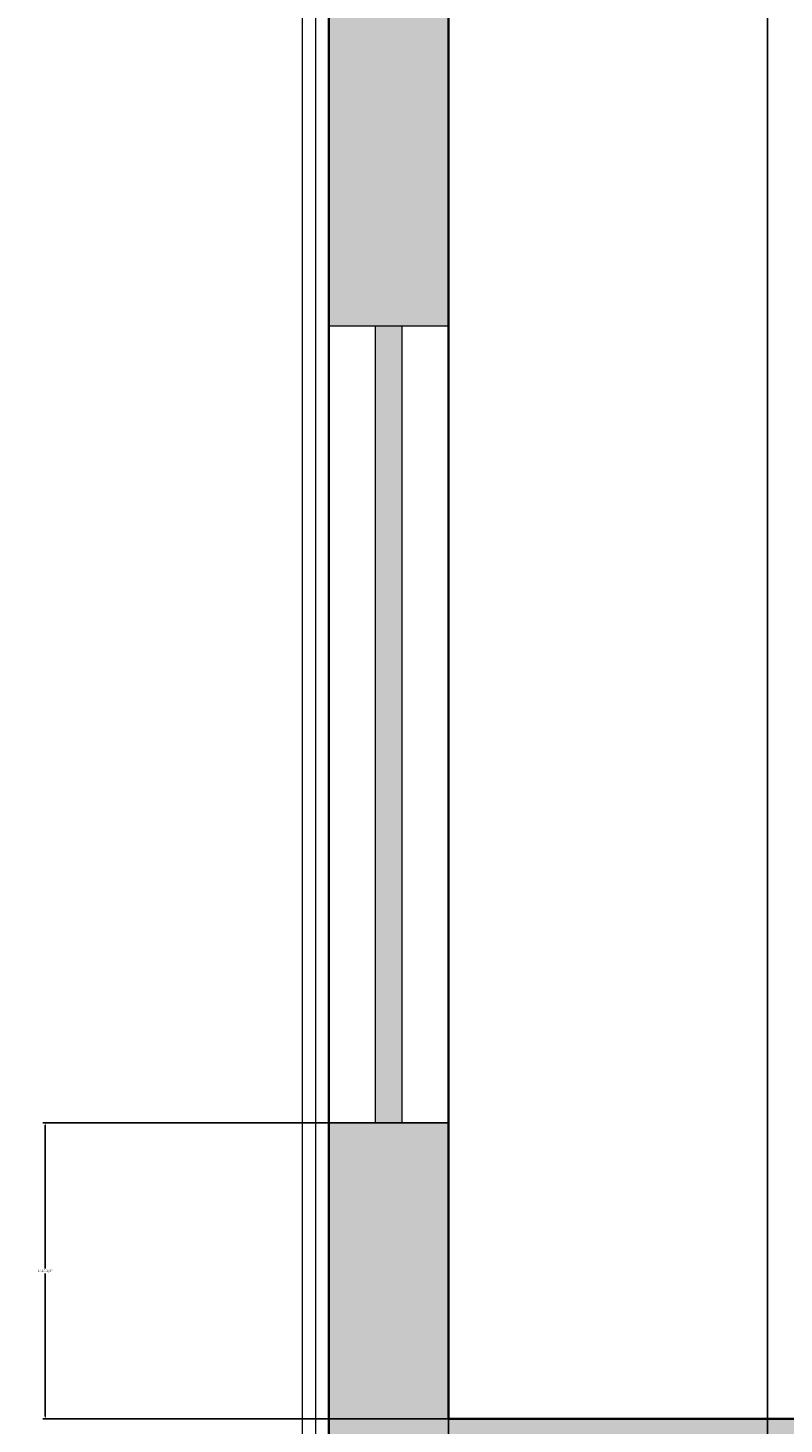
# Model space of a CAD drawing. Units: inches. Extents: x 311 to 815, y -527 to 136.
# Tile 3 of 21: x 388 to 445, y -474 to -368. Entities that reach past the tile are written whole.
import ezdxf

# ---------------------------------------------------------------- set-up
doc = ezdxf.new("R2010")
doc.units = ezdxf.units.IN
doc.header["$MEASUREMENT"] = 0
for name, color, linetype, lineweight in [('A-ANNO-DIMS', 1, 'Continuous', 18), ('A-FLOR-EDGE', 1, 'Continuous', 18), ('A-GLAZ-PATT', 5, 'Continuous', 13), ('A-WALL-PATT', 242, 'Continuous', 13), ('wall', 1, 'Continuous', 35), ('win', 5, 'Continuous', 18)]:
    doc.layers.add(name, color=color, linetype=linetype, lineweight=lineweight)
doc.styles.get("Standard").update_dxf_attribs({"font": 'arial.ttf'})
doc.dimstyles.get("Standard").update_dxf_attribs({"dimtxt": 0.18, "dimasz": 0.18, "dimexe": 0.18, "dimexo": 0.0625, "dimgap": 0.09, "dimtad": 0, "dimtih": 1, "dimtoh": 1, "dimdec": 1, "dimzin": 0, "dimdsep": 46, "dimlunit": 4, "dimtxsty": 'Standard', "dimcen": 0.09, "dimadec": 0, "dimazin": 0, "dimtfac": 1, "dimtdec": 1, "dimtofl": 0, "dimtmove": 0, "dimatfit": 3, "dimfxl": 1, "dimtolj": 1, "dimtzin": 0, "dimarcsym": 0})

# ---------------------------------------------------------------- blocks, each defined once
blk = doc.blocks.new('_ArchTick')
at = {"color": 0, "linetype": 'ByBlock', "const_width": 0.15}
blk.add_lwpolyline([(-0.5, -0.5), (0.5, 0.5)], dxfattribs=at)
blk = doc.blocks.new('_Oblique')
at = {"color": 0, "linetype": 'ByBlock', "lineweight": -2}
blk.add_line((-0.5, -0.5), (0.5, 0.5), dxfattribs=at)
blk = doc.blocks.new('*D3')
at = {"layer": 'A-ANNO-DIMS', "color": 0, "lineweight": -2, "transparency": 16777216}
for p, q in [((377.54, 21.87), (377.54, -221.61)), ((377.54, -482.13), (377.54, -238.65))]:
    blk.add_line(p, q, dxfattribs=at)
at = {"layer": 'Defpoints', "color": 0, "transparency": 16777216}
for p in [(410.32, 21.87), (377.54, -482.13), (410.32, -482.13)]:
    blk.add_point(p, dxfattribs=at)
at = {"layer": 'A-ANNO-DIMS', "color": 0, "lineweight": -2, "transparency": 16777216, "xscale": 9, "yscale": 9, "zscale": 9}
for name, p, rotation in [('_ArchTick', (377.54, 21.87), 90), ('_Oblique', (377.54, -482.13), 270)]:
    blk.add_blockref(name, p, dxfattribs=dict(at, rotation=rotation))
at = {"layer": 'A-ANNO-DIMS', "color": 0, "transparency": 16777216, "insert": (377.54, -230.13), "char_height": 9, "attachment_point": 5}
blk.add_mtext("\\A1;42'", dxfattribs=at)
blk = doc.blocks.new('WIN-60IN')
for p, q in [((9, 60), (0, 60)), ((3.5, 0), (3.5, 60)), ((5.5, 0), (5.5, 60)), ((9, 0), (0, 0))]:
    blk.add_line(p, q)
blk = doc.blocks.new('*D44')
at = {"layer": 'A-ANNO-DIMS', "color": 0, "lineweight": -2, "transparency": 16777216}
for p, q in [((419.26, -450.84), (388.79, -450.84)), ((388.97, -451.02), (388.97, -461.8)), ((388.97, -472.95), (388.97, -462.17)), ((419.26, -473.13), (388.79, -473.13))]:
    blk.add_line(p, q, dxfattribs=at)
at = {"layer": 'A-ANNO-DIMS', "color": 0, "transparency": 16777216}
for points in [[(388.94, -451.02), (389, -451.02), (388.97, -450.84)], [(388.94, -472.95), (389, -472.95), (388.97, -473.13)]]:
    blk.add_solid(points, dxfattribs=at)
at = {"layer": 'Defpoints', "color": 0, "transparency": 16777216}
for p in [(388.97, -450.84), (419.32, -450.84), (419.32, -473.13)]:
    blk.add_point(p, dxfattribs=at)
at = {"layer": 'A-ANNO-DIMS', "color": 0, "transparency": 16777216, "insert": (388.97, -461.98), "char_height": 0.18, "attachment_point": 5}
blk.add_mtext('\\A1;1\'-10 1/2"', dxfattribs=at)
blk = doc.blocks.new('*D54')
at = {"layer": 'A-ANNO-DIMS', "color": 0, "lineweight": -2, "transparency": 16777216}
for p, q in [((419.32, -335.63), (419.32, -526.66)), ((443.32, -348.19), (443.32, -526.66)), ((419.5, -526.48), (430.99, -526.48)), ((443.14, -526.48), (431.65, -526.48))]:
    blk.add_line(p, q, dxfattribs=at)
at = {"layer": 'A-ANNO-DIMS', "color": 0, "transparency": 16777216}
for points in [[(419.5, -526.45), (419.5, -526.51), (419.32, -526.48)], [(443.14, -526.45), (443.14, -526.51), (443.32, -526.48)]]:
    blk.add_solid(points, dxfattribs=at)
at = {"layer": 'Defpoints', "color": 0, "transparency": 16777216}
for p in [(419.32, -335.57), (443.32, -348.13), (443.32, -526.48)]:
    blk.add_point(p, dxfattribs=at)
at = {"layer": 'A-ANNO-DIMS', "color": 0, "transparency": 16777216, "insert": (431.32, -526.48), "char_height": 0.18, "attachment_point": 5}
blk.add_mtext('\\A1;2\'-0"', dxfattribs=at)

msp = doc.modelspace()

# ---------------------------------------------------------------- hatches: boundary and pattern name
at = {"layer": 'A-GLAZ-PATT'}
h = msp.add_hatch(color=256, dxfattribs=at)
h.dxf.hatch_style = 1
h.paths.add_polyline_path([(415.82, -202.13), (413.82, -202.13), (413.82, -262.13), (415.82, -262.13)])
h.paths.add_polyline_path([(415.82, -390.84), (413.82, -390.84), (413.82, -450.84), (415.82, -450.84)])
h.paths.add_polyline_path([(415.82, -311.57), (413.82, -311.57), (413.82, -335.57), (415.82, -335.57)])
h.paths.add_polyline_path([(509.32, -476.63), (449.32, -476.63), (449.32, -478.63), (509.32, -478.63)])
h.paths.add_polyline_path([(606.82, -476.63), (582.82, -476.63), (582.82, -478.63), (606.82, -478.63)])
h.paths.add_polyline_path([(678.82, -476.63), (654.82, -476.63), (654.82, -478.63), (678.82, -478.63)])
h.paths.add_polyline_path([(718.82, -385.13), (716.82, -385.13), (716.82, -445.13), (718.82, -445.13)])
h.paths.add_polyline_path([(718.82, -262.63), (716.82, -262.63), (716.82, -322.63), (718.82, -322.63)])
h.paths.add_polyline_path([(718.82, -140.13), (716.82, -140.13), (716.82, -200.13), (718.82, -200.13)])
h.paths.add_polyline_path([(718.82, -18.13), (716.82, -18.13), (716.82, -42.13), (718.82, -42.13)])
h.paths.add_polyline_path([(686.82, 18.37), (626.82, 18.37), (626.82, 16.37), (686.82, 16.37)])
h.paths.add_polyline_path([(581.82, 18.37), (557.82, 18.37), (557.82, 16.37), (581.82, 16.37)])
h.paths.add_polyline_path([(509.32, 18.37), (449.32, 18.37), (449.32, 16.37), (509.32, 16.37)])
at = {"layer": 'A-WALL-PATT'}
h = msp.add_hatch(color=256, dxfattribs=at)
h.dxf.hatch_style = 1
h.paths.add_polyline_path([(557.82, 21.87), (509.32, 21.87), (509.32, 12.87), (539.32, 12.87), (539.32, -112.13), (548.32, -112.13), (548.32, -58.63), (557.82, -58.63), (557.82, -49.63), (548.32, -49.63), (548.32, 12.87), (557.82, 12.87)])
h.paths.add_polyline_path([(449.32, 21.87), (410.32, 21.87), (410.32, -15.13), (419.32, -15.13), (419.32, 12.87), (449.32, 12.87)])
h.paths.add_polyline_path([(626.82, 21.87), (581.82, 21.87), (581.82, 12.87), (591.32, 12.87), (591.32, -49.63), (581.82, -49.63), (581.82, -58.63), (591.32, -58.63), (591.32, -112.13), (600.32, -112.13), (600.32, 12.87), (626.82, 12.87)])
h.paths.add_polyline_path([(722.32, 21.87), (686.82, 21.87), (686.82, 12.87), (713.32, 12.87), (713.32, -18.13), (722.32, -18.13)])
h.paths.add_polyline_path([(722.32, -42.13), (713.32, -42.13), (713.32, -73.13), (722.32, -73.13)])
h.paths.add_polyline_path([(501.32, -103.13), (419.32, -103.13), (419.32, -75.13), (410.32, -75.13), (410.32, -126.63), (419.32, -126.63), (419.32, -112.13), (492.32, -112.13), (492.32, -143.13), (501.32, -143.13)])
h.paths.add_polyline_path([(548.32, -165.13), (419.32, -165.13), (419.32, -150.63), (410.32, -150.63), (410.32, -202.13), (419.32, -202.13), (419.32, -174.13), (548.32, -174.13)])
h.paths.add_polyline_path([(722.32, -103.13), (636.32, -103.13), (636.32, -112.13), (713.32, -112.13), (713.32, -140.13), (722.32, -140.13)])
h.paths.add_polyline_path([(548.32, -210.13), (539.32, -210.13), (539.32, -290.13), (419.32, -290.13), (419.32, -262.13), (410.32, -262.13), (410.32, -311.57), (419.32, -311.57), (419.32, -299.13), (469.32, -299.13), (469.32, -348.13), (443.32, -348.13), (443.32, -357.13), (478.32, -357.13), (478.32, -299.13), (548.32, -299.13)])
h.paths.add_polyline_path([(722.32, -200.13), (713.32, -200.13), (713.32, -228.13), (609.32, -228.13), (609.32, -237.13), (713.32, -237.13), (713.32, -262.63), (722.32, -262.63)])
h.paths.add_polyline_path([(722.32, -322.63), (713.32, -322.63), (713.32, -348.13), (633.32, -348.13), (633.32, -357.13), (713.32, -357.13), (713.32, -385.13), (722.32, -385.13)])
h.paths.add_polyline_path([(419.32, -335.57), (410.32, -335.57), (410.32, -390.84), (419.32, -390.84)])
h.paths.add_polyline_path([(419.32, -450.84), (410.32, -450.84), (410.32, -482.13), (449.32, -482.13), (449.32, -473.13), (419.32, -473.13)])
h.paths.add_polyline_path([(582.82, -473.13), (548.32, -473.13), (548.32, -348.13), (539.32, -348.13), (539.32, -473.13), (509.32, -473.13), (509.32, -482.13), (582.82, -482.13)])
h.paths.add_polyline_path([(722.32, -445.13), (713.32, -445.13), (713.32, -473.13), (678.82, -473.13), (678.82, -482.13), (722.32, -482.13)])

# ---------------------------------------------------------------- linework, layer by layer
at = {"layer": 'A-FLOR-EDGE'}
for p, q in [((408.32, -484.13), (408.32, 23.87)), ((409.32, -483.13), (409.32, 22.87))]:
    msp.add_line(p, q, dxfattribs=at)
at = {"layer": 'wall'}
for p, q in [((410.32, -482.13), (410.32, 21.87)), ((419.32, -473.13), (419.32, -299.13)), ((419.32, -473.13), (539.32, -473.13))]:
    msp.add_line(p, q, dxfattribs=at)

# ---------------------------------------------------------------- block references
at = {"layer": 'win'}
msp.add_blockref('WIN-60IN', (410.32, -450.84), dxfattribs=at)

# ---------------------------------------------------------------- dimensions: what is measured, and where the dimension line sits
at = {"layer": 'A-ANNO-DIMS'}
for base, p1, p2, override, picture, middle in [((377.54, -482.13), (410.32, 21.87), (410.32, -482.13), {"dimtxt": 9, "dimasz": 9, "dimgap": 4, "dimblk1": 'ArchTick', "dimblk2": 'Oblique', "dimsah": 1, "dimse1": 1, "dimse2": 1, "dimclrd": 0, "dimclre": 0, "dimclrt": 0}, '*D3', (377.54, -230.13)), ((388.97, -450.84), (419.32, -473.13), (419.32, -450.84), {"dimdec": 1, "dimlfac": 1, "dimrnd": 0, "dimzin": 1, "dimdsep": 46, "dimlunit": 4, "dimfrac": 2}, '*D44', (388.97, -461.98))]:
    dim = msp.add_linear_dim(base=base, p1=p1, p2=p2, angle=90, dimstyle='Standard', override=override, dxfattribs=at)
    dim.commit()
    dim.dimension.update_dxf_attribs({"geometry": picture, "text_midpoint": middle})
dim = msp.add_linear_dim(base=(443.32, -526.48), p1=(419.32, -335.57), p2=(443.32, -348.13), dimstyle='Standard', override={"dimdec": 1, "dimlfac": 1, "dimrnd": 0, "dimzin": 1, "dimdsep": 46, "dimlunit": 4, "dimfrac": 2}, dxfattribs=at)
dim.commit()
dim.dimension.update_dxf_attribs({"geometry": '*D54', "text_midpoint": (431.32, -526.48)})

doc.saveas('drawing.dxf')
